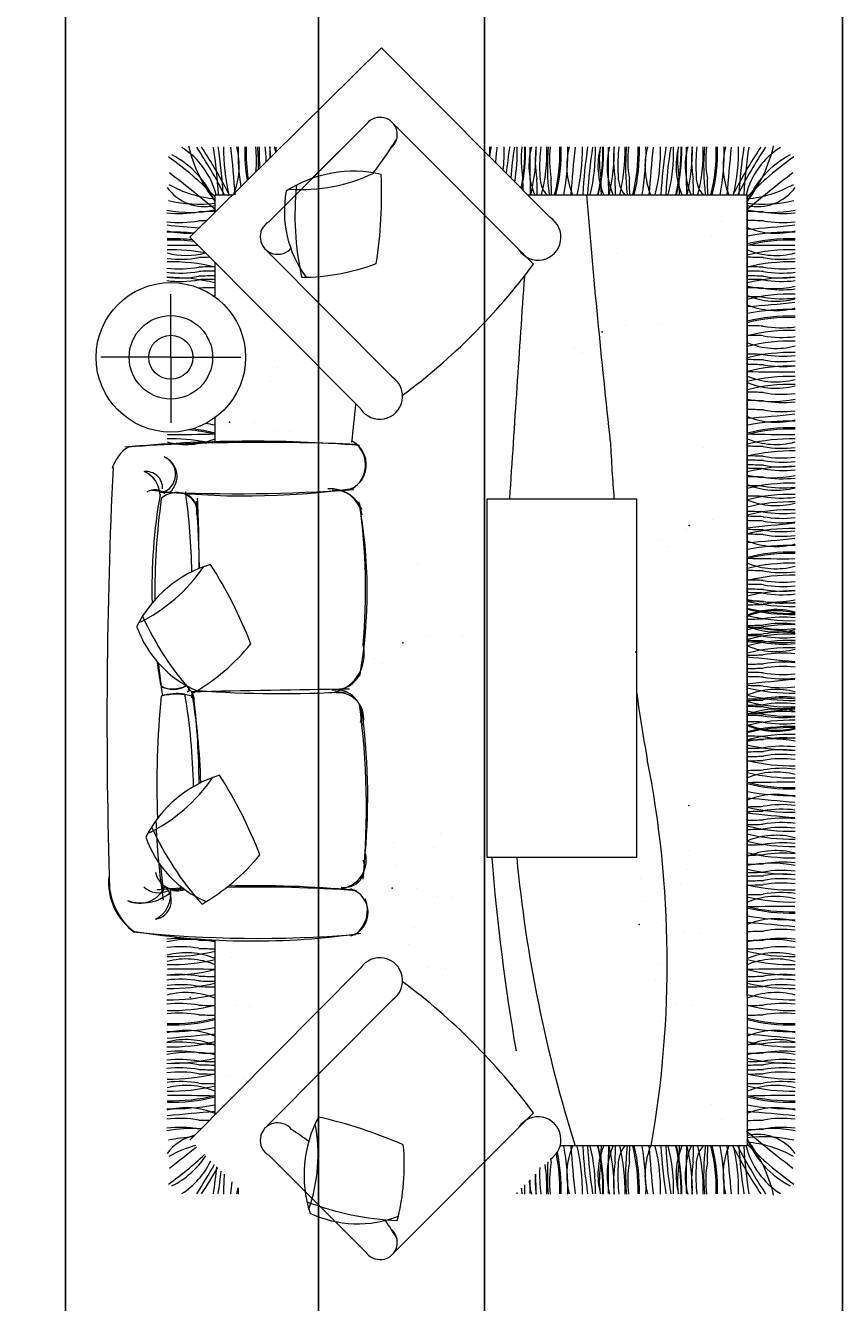
# Model space of a CAD drawing. Units: inches. Extents: x 338 to 1188, y -996 to 127.
# Tile 5 of 15: x 608 to 702, y -386 to -240. Entities that reach past the tile are written whole.
import ezdxf

# ---------------------------------------------------------------- set-up
doc = ezdxf.new("R2010")
doc.units = ezdxf.units.IN
doc.header["$MEASUREMENT"] = 0
doc.layers.add('A-ANNO-DIMS', color=5, linetype='Continuous', lineweight=18)
doc.layers.add('furniture', color=50, linetype='Continuous', lineweight=13, transparency=0.8)
doc.styles.get("Standard").update_dxf_attribs({"font": 'arial.ttf'})
doc.dimstyles.get("Standard").update_dxf_attribs({"dimtxt": 0.18, "dimasz": 0.18, "dimexe": 0.18, "dimexo": 0.0625, "dimgap": 0.09, "dimtad": 0, "dimtih": 1, "dimtoh": 1, "dimdec": 1, "dimzin": 0, "dimdsep": 46, "dimlunit": 4, "dimtxsty": 'Standard', "dimcen": 0.09, "dimadec": 0, "dimazin": 0, "dimtfac": 1, "dimtdec": 1, "dimtofl": 0, "dimtmove": 0, "dimatfit": 3, "dimfxl": 1, "dimtolj": 1, "dimtzin": 0, "dimarcsym": 0})

# ---------------------------------------------------------------- blocks, each defined once
blk = doc.blocks.new('*D31')
at = {"layer": 'A-ANNO-DIMS', "color": 0, "lineweight": -2, "transparency": 16777216}
for p, q in [((641.96, -149.3), (641.96, -968.86)), ((701.96, -149.3), (701.96, -968.86)), ((642.14, -968.68), (671.63, -968.68)), ((701.78, -968.68), (672.29, -968.68))]:
    blk.add_line(p, q, dxfattribs=at)
at = {"layer": 'A-ANNO-DIMS', "color": 0, "transparency": 16777216}
for points in [[(642.14, -968.65), (642.14, -968.71), (641.96, -968.68)], [(701.78, -968.65), (701.78, -968.71), (701.96, -968.68)]]:
    blk.add_solid(points, dxfattribs=at)
at = {"layer": 'Defpoints', "color": 0, "transparency": 16777216}
for p in [(641.96, -149.23), (701.96, -149.23), (701.96, -968.68)]:
    blk.add_point(p, dxfattribs=at)
at = {"layer": 'A-ANNO-DIMS', "color": 0, "transparency": 16777216, "insert": (671.96, -968.68), "char_height": 0.18, "attachment_point": 5}
blk.add_mtext('\\A1;5\'-0"', dxfattribs=at)
blk = doc.blocks.new('*D34')
at = {"layer": 'A-ANNO-DIMS', "color": 0, "lineweight": -2, "transparency": 16777216}
for p, q in [((612.96, -615.67), (612.96, 67.25)), ((613.14, 67.07), (636.63, 67.07)), ((660.78, 67.07), (637.3, 67.07)), ((660.96, -615.67), (660.96, 67.25))]:
    blk.add_line(p, q, dxfattribs=at)
at = {"layer": 'A-ANNO-DIMS', "color": 0, "transparency": 16777216}
for points in [[(613.14, 67.1), (613.14, 67.04), (612.96, 67.07)], [(660.78, 67.1), (660.78, 67.04), (660.96, 67.07)]]:
    blk.add_solid(points, dxfattribs=at)
at = {"layer": 'Defpoints', "color": 0, "transparency": 16777216}
for p in [(660.96, 67.07), (612.96, -615.73), (660.96, -615.73)]:
    blk.add_point(p, dxfattribs=at)
at = {"layer": 'A-ANNO-DIMS', "color": 0, "transparency": 16777216, "insert": (636.96, 67.07), "char_height": 0.18, "attachment_point": 5}
blk.add_mtext('\\A1;4\'-0"', dxfattribs=at)
blk = doc.blocks.new('*D48')
at = {"layer": 'A-ANNO-DIMS', "color": 0, "lineweight": -2, "transparency": 16777216}
for p, q in [((596.96, -615.67), (596.96, 67.25)), ((597.14, 67.07), (604.64, 67.07)), ((612.78, 67.07), (605.28, 67.07)), ((612.96, -615.67), (612.96, 67.25))]:
    blk.add_line(p, q, dxfattribs=at)
at = {"layer": 'A-ANNO-DIMS', "color": 0, "transparency": 16777216}
for points in [[(597.14, 67.1), (597.14, 67.04), (596.96, 67.07)], [(612.78, 67.1), (612.78, 67.04), (612.96, 67.07)]]:
    blk.add_solid(points, dxfattribs=at)
at = {"layer": 'Defpoints', "color": 0, "transparency": 16777216}
for p in [(612.96, 67.07), (596.96, -615.73), (612.96, -615.73)]:
    blk.add_point(p, dxfattribs=at)
at = {"layer": 'A-ANNO-DIMS', "color": 0, "transparency": 16777216, "insert": (604.96, 67.07), "char_height": 0.18, "attachment_point": 5}
blk.add_mtext('\\A1;1\'-4"', dxfattribs=at)

msp = doc.modelspace()

# ---------------------------------------------------------------- linework, layer by layer
at = {"layer": 'furniture'}
for p, q in [((627.21, -264.17), (649.14, -242.51)), ((649.14, -242.51), (668.47, -261.94)), ((636.25, -262.43), (647.5, -251.17)), ((641.22, -257.45), (647.5, -251.17)), ((666.56, -267.29), (650.39, -251.05)), ((664.92, -256.42), (664.92, -256.42)), ((664.96, -255.9), (664.96, -255.9)), ((673.87, -256.42), (673.87, -256.42)), ((673.91, -255.9), (673.91, -255.9)), ((682.82, -256.42), (682.82, -256.42)), ((682.86, -255.9), (682.86, -255.9)), ((630.09, -261.32), (630.09, -259.35)), ((630.09, -259.35), (632.09, -259.35)), ((665.89, -259.35), (691.05, -259.35)), ((691.05, -351.03), (691.05, -259.35)), ((691.05, -259.35), (691.05, -368.24)), ((628.37, -261.08), (628.37, -261.08)), ((628.37, -261.08), (628.37, -261.08)), ((628.37, -261.08), (628.37, -261.08)), ((636.25, -262.43), (638.05, -260.62)), ((692.76, -261.08), (692.76, -261.08)), ((692.76, -261.08), (692.76, -261.08)), ((692.76, -261.08), (692.76, -261.08)), ((628.7, -262.4), (628.7, -262.4)), ((628.7, -262.4), (628.7, -262.4)), ((628.7, -262.4), (628.7, -262.4)), ((688.07, -262.43), (688.07, -262.43)), ((692.44, -262.4), (692.44, -262.4)), ((692.44, -262.4), (692.44, -262.4)), ((692.44, -262.4), (692.44, -262.4)), ((627.21, -264.17), (646.78, -283.86)), ((686.91, -264.07), (686.91, -264.07)), ((635.85, -265.56), (650.41, -280.23)), ((676.07, -266.04), (676.07, -266.04)), ((630.09, -271.04), (630.09, -267.07)), ((625.03, -277.94), (625.03, -270.73)), ((677.16, -274.29), (677.16, -274.29)), ((681.22, -274.23), (681.22, -274.23)), ((674.17, -275.48), (674.17, -275.48)), ((671.23, -276.8), (671.23, -276.8)), ((671.23, -276.8), (671.23, -276.8)), ((672.13, -277.39), (672.13, -277.39)), ((672.13, -277.39), (672.13, -277.39)), ((625.03, -277.94), (617.01, -277.94)), ((625.03, -277.94), (633.05, -277.94)), ((625.03, -277.94), (625.03, -285.44)), ((637.29, -279.12), (637.29, -279.12)), ((636.5, -280.74), (636.5, -280.74)), ((630.09, -287.6), (630.09, -284.85)), ((631.37, -285.76), (631.37, -285.76)), ((634.56, -285.44), (634.56, -285.44)), ((636.93, -286.29), (636.93, -286.29)), ((638.59, -286.41), (638.59, -286.41)), ((686.04, -288.22), (686.04, -288.22)), ((661.25, -335.22), (661.25, -294.13)), ((661.25, -294.13), (678.37, -294.13)), ((678.37, -294.13), (678.37, -335.22)), ((687.13, -296.47), (687.13, -296.47)), ((691.19, -296.41), (691.19, -296.41)), ((684.14, -297.65), (684.14, -297.65)), ((681.2, -298.97), (681.2, -298.97)), ((681.2, -298.97), (681.2, -298.97)), ((682.09, -299.57), (682.09, -299.57)), ((682.09, -299.57), (682.09, -299.57)), ((653.25, -301.69), (653.25, -301.69)), ((692.76, -306.07), (692.76, -306.07)), ((692.76, -306.19), (692.76, -306.19)), ((654.33, -309.94), (654.33, -309.94)), ((658.39, -309.88), (658.39, -309.88)), ((692.76, -309.91), (692.76, -309.91)), ((651.35, -311.12), (651.35, -311.12)), ((648.41, -312.45), (648.41, -312.45)), ((648.41, -312.45), (648.41, -312.45)), ((649.3, -313.04), (649.3, -313.04)), ((649.3, -313.04), (649.3, -313.04)), ((692.76, -317.69), (692.76, -317.69)), ((692.76, -321.4), (692.76, -321.4)), ((692.76, -321.52), (692.76, -321.52)), ((655.93, -332.46), (655.93, -332.46)), ((650.58, -333.49), (650.58, -333.49)), ((655.15, -334.09), (655.15, -334.09)), ((684.27, -334.39), (684.27, -334.39)), ((650.8, -336.07), (650.8, -336.07)), ((678.37, -335.22), (661.25, -335.22)), ((678.87, -337.66), (678.87, -337.66)), ((684.23, -336.64), (684.23, -336.64)), ((650.01, -339.1), (650.01, -339.1)), ((653.21, -338.79), (653.21, -338.79)), ((683.44, -338.27), (683.44, -338.27)), ((655.58, -339.63), (655.58, -339.63)), ((657.23, -339.76), (657.23, -339.76)), ((679.09, -340.25), (679.09, -340.25)), ((652.89, -343.19), (652.89, -343.19)), ((678.31, -343.28), (678.31, -343.28)), ((681.5, -342.96), (681.5, -342.96)), ((630.09, -364.65), (630.09, -344.66)), ((632.79, -344.99), (632.79, -344.99)), ((683.87, -343.81), (683.87, -343.81)), ((685.53, -343.93), (685.53, -343.93)), ((627.43, -346.02), (627.43, -346.02)), ((652.21, -345.12), (652.21, -345.12)), ((627.21, -367.56), (646.78, -347.86)), ((632, -346.62), (632, -346.62)), ((654.54, -347.81), (654.54, -347.81)), ((656.47, -347.95), (656.47, -347.95)), ((681.18, -347.36), (681.18, -347.36)), ((627.65, -348.6), (627.65, -348.6)), ((680.5, -349.3), (680.5, -349.3)), ((652.67, -349.78), (652.67, -349.78)), ((652.67, -349.78), (652.67, -349.78)), ((626.86, -351.63), (626.86, -351.63)), ((630.06, -351.32), (630.06, -351.32)), ((632.43, -352.16), (632.43, -352.16)), ((634.09, -352.29), (634.09, -352.29)), ((635.85, -366.16), (650.41, -351.5)), ((682.83, -351.98), (682.83, -351.98)), ((684.76, -352.12), (684.76, -352.12)), ((680.97, -353.96), (680.97, -353.96)), ((680.97, -353.96), (680.97, -353.96)), ((629.74, -355.72), (629.74, -355.72)), ((629.06, -357.66), (629.06, -357.66)), ((631.39, -360.34), (631.39, -360.34)), ((633.32, -360.48), (633.32, -360.48)), ((629.53, -362.32), (629.53, -362.32)), ((629.53, -362.32), (629.53, -362.32)), ((686.91, -363.52), (686.91, -363.52)), ((628.7, -365.19), (628.7, -365.19)), ((628.7, -365.19), (628.7, -365.19)), ((628.7, -365.19), (628.7, -365.19)), ((666.56, -364.43), (650.39, -380.67)), ((688.07, -365.16), (688.07, -365.16)), ((692.44, -365.19), (692.44, -365.19)), ((692.44, -365.19), (692.44, -365.19)), ((692.44, -365.19), (692.44, -365.19)), ((628.37, -366.51), (628.37, -366.51)), ((628.37, -366.51), (628.37, -366.51)), ((628.37, -366.51), (628.37, -366.51)), ((692.76, -366.51), (692.76, -366.51)), ((692.76, -366.51), (692.76, -366.51)), ((692.76, -366.51), (692.76, -366.51)), ((691.05, -368.24), (669.63, -368.24)), ((636.25, -369.3), (647.5, -380.55)), ((636.25, -369.3), (640.41, -373.46)), ((673.87, -371.17), (673.87, -371.17)), ((682.82, -371.17), (682.82, -371.17)), ((673.91, -371.69), (673.91, -371.69)), ((682.86, -371.69), (682.86, -371.69)), ((643.84, -376.89), (647.5, -380.55))]:
    msp.add_line(p, q, dxfattribs=at)
for radius in [8.56, 4.78, 2.52]:
    msp.add_circle((625.03, -277.94), radius, dxfattribs=at)
for centre, radius, start, end in [((649, -252.44), 1.97, 310.1092, 139.8908), ((617.94, -233.04), 38.5, 321.8457, 328.9133), ((621.47, -261.52), 9.01, 13.9935, 57.7288), ((642.86, -250.08), 16.22, 192.9523, 218.0769), ((576.59, -287.48), 61.41, 27.2669, 33.1781), ((577.14, -287.47), 61.41, 27.2669, 33.1781), ((570.94, -262.81), 59.64, 3.3644, 8.6229), ((571.49, -262.8), 59.64, 3.3644, 8.6229), ((651.94, -254.34), 20.87, 178.6331, 193.8573), ((389.59, -278.5), 243.57, 4.5146, 5.8017), ((624.31, -256.05), 8.55, 337.3098, 14.8613), ((660.44, -254.32), 27.71, 179.0195, 188.4847), ((654.36, -254.35), 20.87, 178.6331, 189.2236), ((654.51, -254.35), 20.87, 178.6331, 188.8561), ((622.45, -255.33), 12.39, 353.6069, 6.8829), ((606.88, -256.06), 28.19, 359.2987, 4.5064), ((656, -254.35), 20.87, 178.6331, 185.2422), ((616.65, -256.01), 19.31, 1.4332, 6.4413), ((624.08, -255.33), 12.39, 1.3666, 6.8829), ((657.24, -254.34), 20.87, 178.6331, 182.1135), ((628.64, -256.03), 8.55, 10.6792, 14.8613), ((458.45, -255.12), 178.63, 0.2284, 0.3934), ((669.99, -256.05), 8.55, 165.1387, 172.5478), ((633.85, -254.32), 27.71, 358.619, 0.9805), ((904.7, -278.5), 243.57, 174.1983, 174.6171), ((642.35, -254.34), 20.87, 353.9229, 1.3669), ((722.8, -262.8), 59.64, 171.3771, 174.3194), ((723.35, -262.81), 59.64, 171.3771, 174.7986), ((643.84, -254.36), 20.87, 350.3159, 1.3669), ((644.71, -254.34), 20.87, 348.2362, 1.3669), ((677.55, -255.34), 12.39, 173.1171, 190.0651), ((644.78, -254.35), 20.87, 348.0993, 1.3669), ((674.6, -256.03), 8.55, 165.1387, 202.6902), ((844.78, -255.12), 178.63, 179.6066, 181.372), ((646, -254.34), 20.87, 346.1427, 1.3669), ((679.16, -255.33), 12.39, 173.1171, 190.0651), ((686.58, -256.01), 19.31, 173.5587, 182.5565), ((647.24, -254.35), 20.87, 346.1427, 1.3669), ((696.35, -256.06), 28.19, 175.4936, 186.6298), ((680.79, -255.33), 12.39, 173.1171, 190.0651), ((648.73, -254.35), 20.87, 346.1427, 1.3669), ((648.88, -254.35), 20.87, 346.1427, 1.3669), ((642.8, -254.32), 27.71, 349.5961, 0.9805), ((678.93, -256.05), 8.55, 165.1387, 202.6902), ((913.65, -278.5), 243.57, 174.1983, 175.4854), ((651.3, -254.34), 20.87, 346.1427, 1.3669), ((731.74, -262.8), 59.64, 171.3771, 176.6356), ((732.3, -262.81), 59.64, 171.3771, 176.6356), ((652.8, -254.36), 20.87, 346.1427, 1.3669), ((653.66, -254.34), 20.87, 346.1427, 1.3669), ((682.5, -256.05), 8.55, 165.1387, 202.6902), ((653.73, -254.35), 20.87, 346.1427, 1.3669), ((686.5, -255.34), 12.39, 173.1171, 190.0651), ((683.55, -256.03), 8.55, 165.1387, 202.6902), ((853.74, -255.12), 178.63, 179.6066, 181.372), ((654.96, -254.34), 20.87, 346.1427, 1.3669), ((688.12, -255.33), 12.39, 173.1171, 190.0651), ((695.54, -256.01), 19.31, 173.5587, 182.5565), ((656.19, -254.35), 20.87, 346.1427, 1.3669), ((705.31, -256.06), 28.19, 175.4936, 186.6298), ((689.75, -255.33), 12.39, 173.1171, 190.0651), ((657.68, -254.35), 20.87, 346.1427, 1.3669), ((657.84, -254.35), 20.87, 346.1427, 1.3669), ((651.75, -254.32), 27.71, 349.5961, 0.9805), ((687.89, -256.05), 8.55, 165.1387, 202.6902), ((922.6, -278.5), 243.57, 174.1983, 175.4854), ((660.25, -254.34), 20.87, 346.1427, 1.3669), ((740.7, -262.8), 59.64, 171.3771, 176.6356), ((741.25, -262.81), 59.64, 171.3771, 176.6356), ((661.74, -254.36), 20.87, 346.1427, 1.3669), ((662.61, -254.34), 20.87, 346.1427, 1.3669), ((691.45, -256.05), 8.55, 165.1387, 202.6902), ((662.68, -254.35), 20.87, 346.1427, 1.3669), ((695.45, -255.34), 12.39, 173.1171, 190.0651), ((692.5, -256.03), 8.55, 165.1387, 202.6902), ((862.68, -255.12), 178.63, 179.6066, 181.372), ((663.9, -254.34), 20.87, 346.1427, 1.3669), ((697.06, -255.33), 12.39, 173.1171, 190.0651), ((704.48, -256.01), 19.31, 173.5587, 182.5565), ((665.14, -254.35), 20.87, 346.1427, 1.3669), ((714.25, -256.06), 28.19, 175.4936, 186.6298), ((698.69, -255.33), 12.39, 173.1171, 190.0651), ((666.63, -254.35), 20.87, 346.1427, 1.3669), ((666.78, -254.35), 20.87, 346.1427, 1.3669), ((660.7, -254.32), 27.71, 349.5961, 0.9805), ((696.83, -256.05), 8.55, 165.1387, 202.6902), ((931.54, -278.5), 243.57, 174.1983, 175.4854), ((744, -287.47), 61.41, 146.8219, 152.7331), ((669.2, -254.34), 20.87, 346.1427, 1.3669), ((744.55, -287.48), 61.41, 146.8219, 152.7331), ((749.64, -262.8), 59.64, 171.3771, 176.6356), ((750.2, -262.81), 59.64, 171.3771, 176.6356), ((699.67, -261.52), 9.01, 122.2712, 166.0065), ((678.27, -250.08), 16.22, 321.9231, 347.0477), ((603.49, -285.02), 36.8, 43.716, 54.6847), ((620.32, -264.15), 10.55, 22.1181, 62.6967), ((700.82, -264.15), 10.55, 117.3033, 157.8819), ((717.65, -285.02), 36.8, 125.3153, 136.284), ((521.87, -390.83), 169.01, 50.1568, 52.4559), ((645.94, -270.78), 14.14, 77.0126, 122.9429), ((640, -239.59), 19.14, 265.9005, 295.6513), ((596.23, -259.24), 52.94, 351.3371, 2.4176), ((671.02, -257.08), 3.73, 176.8256, 218.3436), ((679.98, -257.08), 3.73, 176.8256, 218.3436), ((688.92, -257.08), 3.73, 176.8256, 218.3436), ((799.27, -390.83), 169.01, 127.5441, 129.8432), ((628.91, -255.36), 5.33, 215.9057, 282.8054), ((631.03, -247.3), 12.51, 240.135, 265.7243), ((672.65, -261.68), 33.41, 174.0815, 192.2768), ((527.26, -261.87), 138.16, 1.2535, 1.8109), ((528.87, -261.86), 138.16, 1.0225, 1.8109), ((530.5, -261.86), 138.16, 1.0225, 1.8109), ((536.21, -261.87), 138.16, 1.0225, 1.8109), ((537.83, -261.86), 138.16, 1.0225, 1.8109), ((539.46, -261.86), 138.16, 1.0225, 1.8109), ((545.16, -261.87), 138.16, 1.0225, 1.8109), ((546.77, -261.86), 138.16, 1.0225, 1.8109), ((548.4, -261.86), 138.16, 1.0225, 1.8109), ((690.11, -247.3), 12.51, 274.2757, 299.865), ((692.23, -255.36), 5.33, 257.1946, 324.0943), ((628.22, -245.35), 15.05, 256.7215, 277.1491), ((650.65, -261.22), 12.62, 169.4501, 216.7699), ((1680.39, -176.52), 1011.15, 184.69873, 186.31076), ((692.92, -245.35), 15.05, 262.8509, 283.2785), ((626.07, -249.09), 12.39, 263.1171, 280.0651), ((627.29, -247.47), 13.88, 258.7545, 281.5888), ((632.6, -399.38), 138.16, 91.0225, 91.8109), ((688.54, -399.38), 138.16, 88.1891, 88.9775), ((693.84, -247.47), 13.88, 258.4112, 281.2455), ((695.07, -249.09), 12.39, 259.9349, 276.8829), ((626.06, -250.12), 12.39, 263.1171, 280.0651), ((649.24, -20.47), 243.57, 264.1983, 265.0575), ((632.6, -400.41), 138.16, 91.4616, 91.8109), ((637.26, -264.15), 2, 120.4819, 322.3252), ((667.09, -264.19), 2.63, 213.0924, 58.5307), ((688.54, -400.41), 138.16, 88.1891, 88.9775), ((694.34, -255.18), 8.55, 247.3098, 284.8613), ((671.9, -20.47), 243.57, 274.5146, 275.8017), ((695.07, -250.12), 12.39, 259.9349, 276.8829), ((625.06, -291.32), 27.71, 84.6488, 90.9805), ((626.8, -255.18), 8.55, 255.1387, 276.0041), ((625.1, -285.23), 20.87, 83.2584, 91.3669), ((625.09, -285.39), 20.87, 82.7707, 91.3669), ((696.04, -285.23), 20.87, 88.6331, 103.8573), ((696.04, -285.39), 20.87, 88.6331, 103.8573), ((696.07, -291.32), 27.71, 89.0195, 100.4039), ((625.09, -286.5), 20.87, 79.2534, 91.3669), ((626.79, -257.73), 8.55, 255.1387, 284.8341), ((625.87, -86.49), 178.63, 269.6066, 270.7304), ((695.27, -86.49), 178.63, 268.628, 270.3934), ((694.35, -257.73), 8.55, 247.3098, 284.8613), ((696.05, -286.5), 20.87, 88.6331, 103.8573), ((626.08, -254.33), 12.39, 263.1171, 280.0651), ((625.09, -287.88), 20.87, 76.1427, 91.3669), ((632.61, -404.62), 138.16, 91.2964, 91.8109), ((639.87, -244.04), 24.74, 270.3068, 290.5663), ((608.1, -223.87), 72.82, 306.6613, 323.3951), ((688.53, -404.62), 138.16, 88.1891, 88.9775), ((696.05, -287.88), 20.87, 88.6331, 103.8573), ((695.06, -254.33), 12.39, 259.9349, 276.8829), ((626.07, -255.42), 12.39, 263.1171, 280.0651), ((626.07, -255.91), 12.39, 263.1171, 280.0651), ((626.07, -256.46), 12.39, 263.1171, 280.0651), ((625.08, -289.68), 20.87, 76.1427, 91.3669), ((632.6, -405.71), 138.16, 91.0225, 91.8109), ((632.6, -406.2), 138.16, 91.0225, 91.8109), ((632.6, -406.75), 138.16, 91.0225, 91.8109), ((5549.12, -607.42), 4895.33, 176.03178, 176.33069), ((688.53, -405.71), 138.16, 88.1891, 88.9775), ((688.54, -406.2), 138.16, 88.1891, 88.9775), ((688.54, -406.75), 138.16, 88.1891, 88.9775), ((696.05, -289.68), 20.87, 88.6331, 103.8573), ((695.06, -255.42), 12.39, 259.9349, 276.8829), ((695.07, -255.91), 12.39, 259.9349, 276.8829), ((695.07, -256.46), 12.39, 259.9349, 276.8829), ((626.07, -256.86), 12.39, 263.1171, 280.0651), ((632.6, -407.15), 138.16, 91.0225, 91.8109), ((632.6, -408.11), 138.16, 91.0225, 91.8109), ((688.54, -407.15), 138.16, 88.1891, 88.9775), ((688.54, -408.11), 138.16, 88.1891, 88.9775), ((693.84, -256.2), 13.88, 258.4112, 281.2455), ((695.07, -256.86), 12.39, 259.9349, 276.8829), ((695.07, -257.82), 12.39, 259.9349, 276.8829), ((626.78, -262.98), 8.55, 291.652, 292.6902), ((632.6, -409.14), 138.16, 91.0225, 91.0606), ((688.54, -409.14), 138.16, 88.1891, 88.9775), ((694.34, -264.03), 8.55, 247.3098, 284.8613), ((696.06, -291.57), 20.87, 88.6331, 103.8573), ((694.36, -262.98), 8.55, 247.3098, 284.8613), ((671.9, -29.32), 243.57, 274.5146, 275.8017), ((695.07, -258.85), 12.39, 259.9349, 276.8829), ((696.04, -294.08), 20.87, 88.6331, 103.8573), ((696.04, -294.24), 20.87, 88.6331, 103.8573), ((696.07, -300.17), 27.71, 89.0195, 100.4039), ((688.53, -412.46), 138.16, 88.1891, 88.9775), ((695.06, -262.17), 12.39, 259.9349, 276.8829), ((688.53, -413.56), 138.16, 88.1891, 88.9775), ((696.05, -295.73), 20.87, 88.6331, 103.8573), ((696.06, -296.96), 20.87, 88.6331, 103.8573), ((694.36, -268.37), 8.55, 247.3098, 284.8613), ((695.06, -263.27), 12.39, 259.9349, 276.8829), ((688.52, -415.71), 138.16, 88.1891, 88.9775), ((696.06, -298.26), 20.87, 88.6331, 103.8573), ((695.06, -265.42), 12.39, 259.9349, 276.8829), ((688.54, -416.34), 138.16, 88.1891, 88.9775), ((688.54, -416.89), 138.16, 88.1891, 88.9775), ((696.05, -299.82), 20.87, 88.6331, 103.8573), ((695.07, -266.05), 12.39, 259.9349, 276.8829), ((695.07, -266.6), 12.39, 259.9349, 276.8829), ((648.96, -282.41), 2.62, 213.6335, 56.3665), ((695.27, -100.98), 178.63, 268.628, 270.3934), ((694.35, -272.21), 8.55, 247.3098, 284.8613), ((696.05, -300.99), 20.87, 88.6331, 103.8573), ((688.54, -420.06), 138.16, 88.1891, 88.9775), ((694.34, -272.93), 8.55, 247.3098, 284.8613), ((696.04, -301.92), 20.87, 88.6331, 103.8573), ((695.07, -269.78), 12.39, 259.9349, 276.8829), ((-359.26, -176.52), 1011.15, 353.68924, 353.93736), ((688.54, -421.02), 138.16, 88.1891, 88.9775), ((693.84, -269.12), 13.88, 258.4112, 281.2455), ((695.07, -270.73), 12.39, 259.9349, 276.8829), ((688.54, -422.05), 138.16, 88.1891, 88.9775), ((694.34, -276.83), 8.55, 247.3098, 284.8613), ((671.9, -42.11), 243.57, 274.5146, 275.8017), ((695.07, -271.77), 12.39, 259.9349, 276.8829), ((625.09, -307.03), 20.87, 76.1427, 84.5854), ((625.1, -306.88), 20.87, 76.1427, 83.4467), ((625.06, -312.96), 27.71, 79.5961, 81.862), ((696.04, -306.88), 20.87, 88.6331, 103.8573), ((696.04, -307.03), 20.87, 88.6331, 103.8573), ((696.07, -312.96), 27.71, 89.0195, 100.4039), ((634.36, -441.94), 154.39, 85.4325, 95.431), ((635.72, -514.28), 226.6, 87.3143, 93.933), ((626.79, -279.37), 8.55, 255.1387, 292.6902), ((625.09, -308.15), 20.87, 79.3731, 91.3669), ((625.87, -108.14), 178.63, 269.6066, 271.372), ((644.39, -290.24), 3.03, 284.6379, 64.3095), ((644.1, -290.25), 3.23, 303.041, 46.0653), ((894.28, -277.01), 219.16, 182.7877, 184.4807), ((695.27, -108.14), 178.63, 268.628, 270.3934), ((694.35, -279.37), 8.55, 247.3098, 284.8613), ((696.05, -308.15), 20.87, 88.6331, 103.8573), ((622.46, -291.88), 4.32, 121.8817, 163.9672), ((623.43, -291.34), 2.15, 284.7814, 67.5922), ((623.33, -291.58), 2.41, 312.3134, 67.6102), ((688.53, -426.26), 138.16, 88.1891, 88.9775), ((688.53, -427.36), 138.16, 88.1891, 88.9775), ((696.05, -309.53), 20.87, 88.6331, 103.8573), ((695.06, -275.97), 12.39, 259.9349, 276.8829), ((695.06, -277.07), 12.39, 259.9349, 276.8829), ((1229.86, -319.71), 612.15, 177.2697, 181.7875), ((688.54, -427.85), 138.16, 88.1891, 88.9775), ((688.54, -428.39), 138.16, 88.1891, 88.9775), ((688.54, -428.79), 138.16, 88.1891, 88.9775), ((696.05, -311.32), 20.87, 88.6331, 103.8573), ((695.07, -277.56), 12.39, 259.9349, 276.8829), ((695.07, -278.1), 12.39, 259.9349, 276.8829), ((695.07, -278.51), 12.39, 259.9349, 276.8829), ((622.19, -292.92), 1.9, 358.0108, 96.5585), ((620.89, -293.69), 2.87, 1.184, 67.8216), ((688.54, -429.75), 138.16, 88.1891, 88.9775), ((693.84, -277.85), 13.88, 258.4112, 281.2455), ((696.06, -313.22), 20.87, 88.6331, 103.8573), ((695.07, -279.46), 12.39, 259.9349, 276.8829), ((623.19, -294.72), 1.62, 44.3938, 123.5856), ((633.58, -205.5), 88.31, 262.9836, 277.989), ((684.53, -304.37), 61.67, 169.9466, 181.5903), ((632.28, -95.63), 197.93, 267.5073, 273.9592), ((625.66, -295.95), 2.52, 6.1174, 133.1189), ((626, -295.47), 2, 347.6226, 80.3094), ((540.68, -304.58), 86.78, 1.3731, 7.4472), ((643.33, -296.69), 3.7, 10.9756, 94.9747), ((643.67, -296.58), 3.43, 19.8228, 92.4985), ((688.52, -431.96), 138.16, 88.1891, 88.9775), ((688.54, -430.78), 138.16, 88.1891, 88.9775), ((694.36, -284.62), 8.55, 247.3098, 284.8613), ((696.06, -314.51), 20.87, 88.6331, 103.8573), ((695.07, -280.5), 12.39, 259.9349, 276.8829), ((702.53, -304.94), 79.34, 172.1551, 180.5585), ((509.53, -303.66), 118.78, 0.7456, 4.456), ((480.55, -301.19), 147.71, 359.6386, 2.7653), ((591.12, -304.69), 56.4, 350.0543, 10.4167), ((572.03, -304.61), 75.3, 355.2072, 7.551), ((694.34, -286.37), 8.55, 247.3098, 284.8613), ((696.04, -315.36), 20.87, 88.6331, 103.8573), ((695.06, -281.67), 12.39, 259.9349, 276.8829), ((688.52, -433.73), 138.16, 88.1891, 88.9775), ((688.53, -434.28), 138.16, 88.1891, 88.9775), ((688.54, -434.78), 138.16, 88.1891, 88.9775), ((696.04, -316.27), 20.87, 88.6331, 103.8573), ((695.05, -283.44), 12.39, 259.9349, 276.8829), ((695.06, -283.99), 12.39, 259.9349, 276.8829), ((695.07, -284.49), 12.39, 259.9349, 276.8829), ((688.51, -435.8), 138.16, 88.1891, 88.9775), ((688.52, -436.33), 138.16, 88.1891, 88.9775), ((739.31, -758.16), 463.19, 95.3008, 95.9835), ((696.03, -318.42), 20.87, 88.6331, 103.8573), ((695.04, -285.51), 12.39, 259.9349, 276.8829), ((695.05, -286.04), 12.39, 259.9349, 276.8829), ((694.34, -291.05), 8.55, 247.3098, 284.8613), ((671.9, -56.34), 243.57, 274.5146, 275.8017), ((696.07, -327.19), 27.71, 89.0195, 100.4039), ((695.27, -122.37), 178.63, 268.628, 270.3934), ((696.04, -321.11), 20.87, 88.6331, 103.8573), ((696.04, -321.26), 20.87, 88.6331, 103.8573), ((633.71, -315.17), 14.14, 107.0126, 152.9429), ((612.97, -291.13), 19.14, 295.9005, 325.6513), ((584.89, -330.03), 52.94, 21.3371, 32.4176), ((688.53, -440.49), 138.16, 88.1891, 88.9775), ((694.35, -293.6), 8.55, 247.3098, 284.8613), ((696.05, -322.38), 20.87, 88.6331, 103.8573), ((695.06, -290.2), 12.39, 259.9349, 276.8829), ((688.53, -441.58), 138.16, 88.1891, 88.9775), ((688.54, -442.07), 138.16, 88.1891, 88.9775), ((696.05, -323.76), 20.87, 88.6331, 103.8573), ((695.06, -291.3), 12.39, 259.9349, 276.8829), ((695.07, -291.79), 12.39, 259.9349, 276.8829), ((688.54, -442.62), 138.16, 88.1891, 88.9775), ((688.54, -443.02), 138.16, 88.1891, 88.9775), ((696.05, -325.55), 20.87, 88.6331, 103.8573), ((695.07, -292.33), 12.39, 259.9349, 276.8829), ((695.07, -292.74), 12.39, 259.9349, 276.8829), ((688.52, -168.14), 138.16, 271.0225, 271.8109), ((688.54, -443.98), 138.16, 88.1891, 88.9775), ((696.04, -285.6), 20.87, 256.1427, 271.3669), ((696.04, -286.39), 20.87, 256.1427, 271.3669), ((696.04, -286.51), 20.87, 256.1427, 271.3669), ((694.34, -315.38), 8.55, 75.1387, 112.6902), ((694.34, -315.5), 8.55, 75.1387, 112.6902), ((693.84, -292.08), 13.88, 258.4112, 281.2455), ((695.05, -318.42), 12.39, 83.1171, 100.0651), ((695.07, -293.69), 12.39, 259.9349, 276.8829), ((652.29, -293.94), 33.41, 204.0815, 222.2768), ((688.52, -169.79), 138.16, 271.0225, 271.8109), ((696.06, -287.23), 20.87, 256.1427, 271.3669), ((695.04, -320.8), 12.39, 83.1171, 100.0651), ((695.06, -320.08), 12.39, 83.1171, 100.0651), ((633.01, -304.54), 12.62, 199.4501, 246.7699), ((688.51, -170.51), 138.16, 271.0225, 271.8109), ((688.52, -447.96), 138.16, 88.1891, 88.9775), ((688.54, -446.99), 138.16, 88.1891, 88.9775), ((688.54, -171.53), 138.16, 271.0225, 271.8109), ((739.31, 151.84), 463.19, 264.0165, 264.6992), ((696.04, -330.5), 20.87, 88.6331, 103.8573), ((696.06, -329.42), 20.87, 88.6331, 103.8573), ((694.36, -300.83), 8.55, 247.3098, 284.8613), ((695.05, -297.67), 12.39, 259.9349, 276.8829), ((695.07, -296.7), 12.39, 259.9349, 276.8829), ((695.07, -321.82), 12.39, 83.1171, 100.0651), ((615.08, -295.05), 24.74, 300.3068, 320.5663), ((642.73, -311.94), 4.46, 276.5867, 13.4511), ((688.53, -448.51), 138.16, 88.1891, 88.9775), ((688.52, -448.67), 138.16, 88.1891, 88.9775), ((694.34, -303.09), 8.55, 247.3098, 284.8613), ((696.04, -332.07), 20.87, 88.6331, 103.8573), ((696.06, -331.23), 20.87, 88.6331, 103.8573), ((695.06, -298.22), 12.39, 259.9349, 276.8829), ((695.06, -298.39), 12.39, 259.9349, 276.8829), ((684.53, -304.37), 61.67, 187.803, 190.4557), ((688.51, -173.92), 138.16, 271.0225, 271.8109), ((739.31, 148.44), 463.19, 264.0165, 264.6992), ((695.04, -324.21), 12.39, 83.1171, 100.0651), ((695.07, -325.23), 12.39, 83.1171, 100.0651), ((702.53, -304.94), 79.34, 185.7795, 188.522), ((643.77, -312.77), 3.26, 264.9234, 335.6374), ((688.53, -175.44), 138.16, 271.0225, 271.8109), ((688.53, -452.15), 138.16, 88.1891, 88.9775), ((688.54, -174.94), 138.16, 271.0225, 271.8109), ((695.06, -325.73), 12.39, 83.1171, 100.0651), ((695.06, -301.87), 12.39, 259.9349, 276.8829), ((625.35, -313.1), 2.86, 239.8319, 299.468), ((625.14, -311.68), 4.21, 253.3108, 292.6164), ((540.68, -304.58), 86.78, 352.7245, 352.7726), ((688.51, -453.67), 138.16, 88.1891, 88.9775), ((688.54, -452.65), 138.16, 88.1891, 88.9775), ((739.31, -776.03), 463.19, 95.3008, 95.9835), ((696.04, -295.52), 20.87, 256.1427, 271.3669), ((695.04, -303.38), 12.39, 259.9349, 276.8829), ((695.07, -302.37), 12.39, 259.9349, 276.8829), ((726.88, -326.9), 103.45, 174.3639, 182.1219), ((625.66, -323.59), 7.07, 74.0479, 104.2061), ((625.78, -322.25), 5.81, 81.5362, 108.3493), ((556.66, -328.34), 70.97, 1.0061, 9.6001), ((626.03, -314.7), 1.79, 299.1313, 312.0141), ((637.67, -184.19), 132.26, 265.3655, 265.4784), ((27526.63, -1508420.89), 1508344.52, 91.02115817, 91.0218453), ((480.55, -301.19), 147.71, 353.8872, 354.1215), ((552.71, -328.82), 75.78, 1.6458, 9.5268), ((656.61, -307.96), 30.31, 195.9625, 197.4638), ((532.99, -327.56), 95.28, 0.4949, 6.3291), ((637.67, -184.19), 132.26, 265.8425, 273.2873), ((644.03, -318.89), 2.86, 343.4437, 91.8228), ((644.24, -319.24), 2.88, 342.9316, 95.1092), ((908.76, -283.39), 232.73, 188.119, 190.0442), ((688.52, -178.92), 138.16, 271.0225, 271.8109), ((688.53, -179.09), 138.16, 271.0225, 271.8109), ((694.34, -324.51), 8.55, 75.1387, 112.6902), ((696.06, -296.36), 20.87, 256.1427, 271.3669), ((695.06, -329.2), 12.39, 83.1171, 100.0651), ((695.06, -329.37), 12.39, 83.1171, 100.0651), ((558.01, -329.61), 89.42, 354.8245, 7.7148), ((571.86, -328.22), 75.72, 355.0781, 7.695), ((688.52, -179.63), 138.16, 271.0225, 271.8109), ((688.54, -456.06), 138.16, 88.1891, 88.9775), ((688.54, -180.6), 138.16, 271.0225, 271.8109), ((739.31, -779.44), 463.19, 95.3008, 95.9835), ((696.04, -297.1), 20.87, 256.1427, 271.3669), ((694.36, -326.76), 8.55, 75.1387, 112.6902), ((696.06, -298.17), 20.87, 256.1427, 271.3669), ((695.05, -329.92), 12.39, 83.1171, 100.0651), ((695.07, -305.77), 12.39, 259.9349, 276.8829), ((695.07, -330.89), 12.39, 83.1171, 100.0651), ((688.51, -457.08), 138.16, 88.1891, 88.9775), ((688.52, -457.8), 138.16, 88.1891, 88.9775), ((694.34, -312.09), 8.55, 247.3098, 284.8613), ((694.34, -312.21), 8.55, 247.3098, 284.8613), ((696.06, -340.36), 20.87, 88.6331, 103.8573), ((695.04, -306.79), 12.39, 259.9349, 276.8829), ((695.06, -307.52), 12.39, 259.9349, 276.8829), ((688.52, -459.45), 138.16, 88.1891, 88.9775), ((696.04, -341.08), 20.87, 88.6331, 103.8573), ((696.04, -341.2), 20.87, 88.6331, 103.8573), ((696.04, -341.99), 20.87, 88.6331, 103.8573), ((695.05, -309.17), 12.39, 259.9349, 276.8829), ((695.07, -333.9), 12.39, 83.1171, 100.0651), ((688.54, -184.57), 138.16, 271.0225, 271.8109), ((688.54, -184.97), 138.16, 271.0225, 271.8109), ((688.54, -183.61), 138.16, 271.0225, 271.8109), ((693.84, -335.52), 13.88, 78.7545, 101.5888), ((696.05, -302.04), 20.87, 256.1427, 271.3669), ((695.07, -334.86), 12.39, 83.1171, 100.0651), ((695.07, -335.26), 12.39, 83.1171, 100.0651), ((562.11, -347.29), 119.78, 349.9275, 11.2246), ((688.54, -185.52), 138.16, 271.0225, 271.8109), ((688.53, -186.01), 138.16, 271.0225, 271.8109), ((696.05, -303.84), 20.87, 256.1427, 271.3669), ((695.07, -335.8), 12.39, 83.1171, 100.0651), ((695.06, -336.29), 12.39, 83.1171, 100.0651), ((634.75, -339.3), 14.14, 107.0126, 152.9429), ((585.92, -354.16), 52.94, 21.3371, 32.4176), ((688.53, -187.1), 138.16, 271.0225, 271.8109), ((694.35, -333.99), 8.55, 75.1387, 112.6902), ((696.05, -305.22), 20.87, 256.1427, 271.3669), ((695.06, -337.39), 12.39, 83.1171, 100.0651), ((614.01, -315.26), 19.14, 295.9005, 325.6513), ((695.27, -505.23), 178.63, 89.6066, 91.372), ((696.04, -306.33), 20.87, 256.1427, 271.3669), ((696.04, -306.49), 20.87, 256.1427, 271.3669), ((694.34, -336.54), 8.55, 75.1387, 112.6902), ((696.07, -300.4), 27.71, 259.5961, 270.9805), ((671.9, -571.25), 243.57, 84.1983, 85.4854), ((688.51, -191.8), 138.16, 271.0225, 271.8109), ((688.52, -191.26), 138.16, 271.0225, 271.8109), ((739.31, 130.56), 463.19, 264.0165, 264.6992), ((696.03, -309.17), 20.87, 256.1427, 271.3669), ((695.04, -342.08), 12.39, 83.1171, 100.0651), ((695.05, -341.55), 12.39, 83.1171, 100.0651), ((653.33, -318.07), 33.41, 204.0815, 222.2768), ((709.07, -327.69), 85.83, 182.2017, 188.3067), ((688.53, -193.31), 138.16, 271.0225, 271.8109), ((688.54, -192.81), 138.16, 271.0225, 271.8109), ((696.04, -311.33), 20.87, 256.1427, 271.3669), ((695.06, -343.6), 12.39, 83.1171, 100.0651), ((695.05, -344.15), 12.39, 83.1171, 100.0651), ((695.07, -343.1), 12.39, 83.1171, 100.0651), ((634.05, -328.67), 12.62, 199.4501, 246.7699), ((688.52, -193.86), 138.16, 271.0225, 271.8109), ((696.04, -312.24), 20.87, 256.1427, 271.3669), ((694.34, -341.22), 8.55, 75.1387, 112.6902), ((644.12, -335.51), 3.29, 267.6579, 14.0974), ((688.52, -195.63), 138.16, 271.0225, 271.8109), ((696.06, -313.08), 20.87, 256.1427, 271.3669), ((694.36, -342.97), 8.55, 75.1387, 112.6902), ((696.06, -314.38), 20.87, 256.1427, 271.3669), ((695.06, -345.92), 12.39, 83.1171, 100.0651), ((695.07, -347.1), 12.39, 83.1171, 100.0651), ((726.88, -326.9), 103.45, 185.0871, 186.7491), ((616.12, -319.19), 24.74, 300.3068, 320.5663), ((644.94, -336.35), 2.28, 260.2617, 21.0115), ((909.91, -315.17), 248.94, 184.6196, 189.7513), ((824.58, -319.98), 160.66, 185.4421, 197.4799), ((688.54, -196.81), 138.16, 271.0225, 271.8109), ((688.54, -197.84), 138.16, 271.0225, 271.8109), ((693.84, -349.74), 13.88, 78.7545, 101.5888), ((695.07, -348.13), 12.39, 83.1171, 100.0651), ((624.59, -338.13), 6.69, 173.8792, 237.1093), ((625.66, -336.46), 2.42, 190.6216, 289.193), ((688.54, -198.8), 138.16, 271.0225, 271.8109), ((688.54, -199.2), 138.16, 271.0225, 271.8109), ((696.05, -316.27), 20.87, 256.1427, 271.3669), ((695.07, -349.08), 12.39, 83.1171, 100.0651), ((695.07, -349.49), 12.39, 83.1171, 100.0651), ((695.07, -350.03), 12.39, 83.1171, 100.0651), ((626.1, -337.57), 8.18, 188.6549, 228.7104), ((621.43, -337.27), 3.18, 244.8715, 336.7247), ((621.69, -335.39), 5.03, 251.2473, 311.1348), ((623.63, -336.7), 2.54, 227.7203, 294.4461), ((622.93, -340.16), 2.15, 279.2916, 47.6289), ((621.75, -339.39), 3.28, 297.8433, 9.8684), ((634.54, -464.2), 125.76, 93.7101, 95.0653), ((625.79, -336.85), 2.17, 237.7366, 292.2387), ((635.09, -491.45), 152.85, 93.1908, 93.7892), ((635.09, -491.45), 152.85, 85.8027, 91.3803), ((634.54, -464.2), 125.76, 84.7422, 91.3335), ((644.8, -341.5), 2.82, 287.7157, 72.8428), ((688.54, -199.75), 138.16, 271.0225, 271.8109), ((688.53, -200.24), 138.16, 271.0225, 271.8109), ((696.05, -318.06), 20.87, 256.1427, 271.3669), ((695.06, -350.52), 12.39, 83.1171, 100.0651), ((644.14, -341.26), 3.41, 306.0678, 22.6723), ((688.53, -201.33), 138.16, 271.0225, 271.8109), ((694.35, -348.22), 8.55, 75.1387, 112.6902), ((696.05, -319.44), 20.87, 256.1427, 271.3669), ((695.06, -351.62), 12.39, 83.1171, 100.0651), ((695.27, -519.45), 178.63, 89.6066, 91.372), ((696.04, -320.56), 20.87, 256.1427, 271.3669), ((696.04, -320.71), 20.87, 256.1427, 271.3669), ((696.07, -314.63), 27.71, 259.5961, 270.9805), ((694.34, -350.77), 8.55, 75.1387, 112.6902), ((671.9, -585.48), 243.57, 84.1983, 85.4854), ((695.07, -355.83), 12.39, 83.1171, 100.0651), ((635, -206.2), 138.27, 264.0627, 274.6253), ((634.44, -259.7), 85.07, 260.8079, 278.3514), ((626.07, -356.86), 12.39, 79.9349, 96.8829), ((627.29, -358.47), 13.88, 78.4112, 101.2455), ((632.6, -206.57), 138.16, 268.1891, 268.9775), ((688.54, -205.54), 138.16, 271.0225, 271.8109), ((688.54, -206.57), 138.16, 271.0225, 271.8109), ((693.84, -358.47), 13.88, 78.7545, 101.5888), ((695.07, -356.86), 12.39, 83.1171, 100.0651), ((626.07, -357.81), 12.39, 79.9349, 96.8829), ((625.1, -325.67), 20.87, 268.6331, 283.8573), ((626.8, -354.66), 8.55, 67.3098, 104.8613), ((632.6, -207.53), 138.16, 268.1891, 268.9775), ((688.54, -207.53), 138.16, 271.0225, 271.8109), ((696.04, -325.67), 20.87, 256.1427, 271.3669), ((694.34, -354.66), 8.55, 75.1387, 112.6902), ((695.07, -357.81), 12.39, 83.1171, 100.0651), ((626.79, -355.38), 8.55, 67.3098, 104.8613), ((625.09, -326.61), 20.87, 268.6331, 283.8573), ((648.96, -349.31), 2.62, 303.6335, 146.3665), ((694.35, -355.38), 8.55, 75.1387, 112.6902), ((696.05, -326.61), 20.87, 256.1427, 271.3669), ((625.08, -327.78), 20.87, 268.6331, 283.8573), ((626.07, -360.99), 12.39, 79.9349, 96.8829), ((626.07, -361.54), 12.39, 79.9349, 96.8829), ((625.87, -526.61), 178.63, 88.628, 90.3934), ((632.6, -210.7), 138.16, 268.1891, 268.9775), ((632.6, -211.25), 138.16, 268.1891, 268.9775), ((695.27, -526.61), 178.63, 89.6066, 91.372), ((688.54, -210.7), 138.16, 271.0225, 271.8109), ((688.54, -211.25), 138.16, 271.0225, 271.8109), ((696.05, -327.78), 20.87, 256.1427, 271.3669), ((695.07, -360.99), 12.39, 83.1171, 100.0651), ((695.07, -361.54), 12.39, 83.1171, 100.0651), ((625.08, -329.33), 20.87, 268.6331, 283.8573), ((626.78, -359.22), 8.55, 67.3098, 104.8613), ((626.08, -362.17), 12.39, 79.9349, 96.8829), ((632.61, -211.89), 138.16, 268.1891, 268.9775), ((608.1, -407.85), 72.82, 36.6049, 53.3387), ((688.52, -211.89), 138.16, 271.0225, 271.8109), ((696.06, -329.33), 20.87, 256.1427, 271.3669), ((694.36, -359.22), 8.55, 75.1387, 112.6902), ((695.06, -362.17), 12.39, 83.1171, 100.0651), ((625.08, -330.63), 20.87, 268.6331, 283.8573), ((626.07, -364.32), 12.39, 79.9349, 96.8829), ((625.09, -331.86), 20.87, 268.6331, 283.8573), ((632.6, -214.03), 138.16, 268.1891, 268.9775), ((688.53, -214.03), 138.16, 271.0225, 271.8109), ((696.05, -331.86), 20.87, 256.1427, 271.3669), ((696.06, -330.63), 20.87, 256.1427, 271.3669), ((695.06, -364.32), 12.39, 83.1171, 100.0651), ((626.08, -365.42), 12.39, 79.9349, 96.8829), ((625.09, -333.35), 20.87, 268.6331, 283.8573), ((625.1, -333.51), 20.87, 268.6331, 283.8573), ((632.61, -215.13), 138.16, 268.1891, 268.9775), ((688.53, -215.13), 138.16, 271.0225, 271.8109), ((696.04, -333.35), 20.87, 256.1427, 271.3669), ((696.04, -333.51), 20.87, 256.1427, 271.3669), ((695.06, -365.42), 12.39, 83.1171, 100.0651), ((625.06, -327.42), 27.71, 269.0195, 280.4039), ((626.8, -363.56), 8.55, 67.3098, 104.8613), ((694.34, -363.56), 8.55, 75.1387, 112.6902), ((696.07, -327.42), 27.71, 259.5961, 270.9805), ((626.78, -364.61), 8.55, 67.3098, 104.8613), ((625.08, -336.02), 20.87, 268.6331, 283.8573), ((626.06, -368.74), 12.39, 79.9349, 96.8829), ((649.24, -598.27), 243.57, 94.5146, 95.8017), ((632.6, -218.45), 138.16, 268.1891, 268.9775), ((688.54, -218.45), 138.16, 271.0225, 271.8109), ((694.36, -364.61), 8.55, 75.1387, 112.6902), ((696.06, -336.02), 20.87, 256.1427, 271.3669), ((671.9, -598.27), 243.57, 84.1983, 85.4854), ((695.07, -368.74), 12.39, 83.1171, 100.0651), ((626.07, -369.77), 12.39, 79.9349, 96.8829), ((627.29, -371.39), 13.88, 78.4112, 101.2455), ((625.08, -337.91), 20.87, 268.6331, 283.8573), ((632.6, -219.49), 138.16, 268.1891, 268.9775), ((688.54, -219.49), 138.16, 271.0225, 271.8109), ((693.84, -371.39), 13.88, 78.7545, 101.5888), ((696.05, -337.91), 20.87, 256.1427, 271.3669), ((695.07, -369.77), 12.39, 83.1171, 100.0651), ((626.07, -370.73), 12.39, 79.9349, 96.8829), ((626.07, -371.13), 12.39, 79.9349, 96.8829), ((626.07, -371.68), 12.39, 79.9349, 96.8829), ((632.6, -220.44), 138.16, 268.1891, 268.9775), ((632.6, -220.84), 138.16, 268.1891, 268.9775), ((632.6, -221.39), 138.16, 268.1891, 268.9775), ((688.54, -220.44), 138.16, 271.0225, 271.8109), ((688.54, -220.84), 138.16, 271.0225, 271.8109), ((688.54, -221.39), 138.16, 271.0225, 271.8109), ((695.07, -370.73), 12.39, 83.1171, 100.0651), ((695.07, -371.13), 12.39, 83.1171, 100.0651), ((695.07, -371.68), 12.39, 83.1171, 100.0651), ((626.07, -372.17), 12.39, 79.9349, 96.8829), ((625.09, -339.71), 20.87, 268.6331, 283.8573), ((626.08, -373.26), 12.39, 79.9349, 96.8829), ((632.6, -221.88), 138.16, 268.1891, 268.9775), ((632.61, -222.97), 138.16, 268.1891, 268.9775), ((688.53, -221.88), 138.16, 271.0225, 271.8109), ((688.53, -222.97), 138.16, 271.0225, 271.8109), ((696.05, -339.71), 20.87, 256.1427, 271.3669), ((695.06, -372.17), 12.39, 83.1171, 100.0651), ((695.06, -373.26), 12.39, 83.1171, 100.0651), ((626.79, -369.86), 8.55, 67.3098, 104.8613), ((625.09, -341.09), 20.87, 268.6331, 283.8573), ((625.09, -342.2), 20.87, 268.6331, 283.8573), ((625.87, -541.1), 178.63, 88.628, 90.3934), ((695.27, -541.1), 178.63, 89.6066, 91.372), ((694.35, -369.86), 8.55, 75.1387, 112.6902), ((696.05, -341.09), 20.87, 256.1427, 271.3669), ((696.04, -342.2), 20.87, 256.1427, 271.3669), ((625.06, -336.27), 27.71, 269.0195, 280.4039), ((625.1, -342.36), 20.87, 268.6331, 283.8573), ((626.8, -372.41), 8.55, 67.3098, 104.8613), ((694.34, -372.41), 8.55, 75.1387, 112.6902), ((696.04, -342.36), 20.87, 256.1427, 271.3669), ((696.07, -336.27), 27.71, 259.5961, 270.9805), ((626.06, -377.47), 12.39, 79.9349, 96.8829), ((649.24, -607.12), 243.57, 94.5146, 95.8017), ((632.6, -227.18), 138.16, 268.1891, 268.6709), ((654.42, -371.57), 14.14, 152.0126, 197.9429), ((630.4, -416.6), 52.94, 66.3371, 77.4176), ((667.09, -367.53), 2.63, 301.4693, 146.9076), ((688.54, -227.18), 138.16, 271.0225, 271.8109), ((671.9, -607.12), 243.57, 84.1983, 85.4854), ((695.07, -377.47), 12.39, 83.1171, 100.0651), ((626.07, -378.5), 12.39, 79.9349, 96.8829), ((627.29, -380.12), 13.88, 85.1756, 101.2455), ((637.26, -367.58), 2, 37.6748, 239.5181), ((617.94, -398.68), 38.5, 53.5454, 57.1144), ((622.75, -369.23), 19.14, 340.9005, 10.6513), ((799.27, -236.77), 169.01, 230.1568, 232.4559), ((688.54, -228.22), 138.16, 271.0225, 271.8109), ((692.23, -372.24), 5.33, 35.9057, 102.8054), ((693.84, -380.12), 13.88, 78.7545, 101.5888), ((695.07, -378.5), 12.39, 83.1171, 100.0651), ((628.91, -372.24), 5.33, 102.9777, 144.0943), ((628.22, -382.24), 15.05, 92.5322, 103.2785), ((631.03, -380.3), 12.51, 104.6792, 119.865), ((521.87, -236.77), 169.01, 307.5441, 308.8901), ((627.03, -370.51), 24.74, 345.3068, 5.5663), ((642.8, -373.27), 27.71, 359.0195, 10.4039), ((678.93, -371.54), 8.55, 157.3098, 194.8613), ((913.65, -349.1), 243.57, 184.5146, 185.8017), ((651.3, -373.25), 20.87, 358.6331, 13.8573), ((731.74, -364.79), 59.64, 183.3644, 188.6229), ((732.3, -364.78), 59.64, 183.3644, 188.6229), ((652.8, -373.23), 20.87, 358.6331, 13.8573), ((653.66, -373.25), 20.87, 358.6331, 13.8573), ((682.5, -371.54), 8.55, 157.3098, 194.8613), ((653.73, -373.24), 20.87, 358.6331, 13.8573), ((536.21, -365.72), 138.16, 358.1891, 358.9775), ((683.55, -371.56), 8.55, 157.3098, 194.8613), ((853.74, -372.47), 178.63, 178.628, 180.3934), ((654.96, -373.26), 20.87, 358.6331, 13.8573), ((537.83, -365.73), 138.16, 358.1891, 358.9775), ((679.98, -370.51), 3.73, 141.6564, 183.1744), ((656.19, -373.25), 20.87, 358.6331, 13.8573), ((705.31, -371.53), 28.19, 173.3702, 184.5064), ((539.46, -365.73), 138.16, 358.1891, 358.9775), ((657.68, -373.24), 20.87, 358.6331, 13.8573), ((657.84, -373.24), 20.87, 358.6331, 13.8573), ((651.75, -373.27), 27.71, 359.0195, 10.4039), ((687.89, -371.54), 8.55, 157.3098, 194.8613), ((922.6, -349.1), 243.57, 184.5146, 185.8017), ((660.25, -373.25), 20.87, 358.6331, 13.8573), ((740.7, -364.79), 59.64, 183.3644, 188.6229), ((741.25, -364.78), 59.64, 183.3644, 188.6229), ((661.74, -373.23), 20.87, 358.6331, 13.8573), ((662.61, -373.25), 20.87, 358.6331, 13.8573), ((691.45, -371.54), 8.55, 157.3098, 194.8613), ((662.68, -373.24), 20.87, 358.6331, 13.8573), ((545.16, -365.72), 138.16, 358.1891, 358.9775), ((692.5, -371.56), 8.55, 157.3098, 194.8613), ((862.68, -372.47), 178.63, 178.628, 180.3934), ((663.9, -373.26), 20.87, 358.6331, 13.8573), ((546.77, -365.73), 138.16, 358.1891, 358.9775), ((688.92, -370.51), 3.73, 141.6564, 183.1744), ((665.14, -373.25), 20.87, 358.6331, 13.8573), ((714.25, -371.53), 28.19, 173.3702, 184.5064), ((548.4, -365.73), 138.16, 358.1891, 358.9775), ((666.63, -373.24), 20.87, 358.6331, 13.8573), ((666.78, -373.24), 20.87, 358.6331, 13.8573), ((660.7, -373.27), 27.71, 359.0195, 10.4039), ((696.83, -371.54), 8.55, 157.3098, 194.8613), ((931.54, -349.1), 243.57, 184.5146, 185.8017), ((744, -340.13), 61.41, 207.2669, 213.1781), ((669.2, -373.25), 20.87, 358.6331, 13.8573), ((744.55, -340.11), 61.41, 207.2669, 213.1781), ((749.64, -364.79), 59.64, 183.3644, 188.6229), ((750.2, -364.78), 59.64, 183.3644, 188.6229), ((699.67, -366.07), 9.01, 193.9935, 237.7288), ((692.92, -382.24), 15.05, 76.7215, 97.1491), ((700.82, -363.44), 10.55, 202.1181, 242.6967), ((678.27, -377.51), 16.22, 12.9523, 38.0769), ((690.11, -380.3), 12.51, 60.135, 85.7243), ((717.65, -342.58), 36.8, 223.716, 234.6847), ((603.49, -342.58), 36.8, 305.3153, 313.6457), ((620.32, -363.44), 10.55, 297.3033, 325.7016), ((530.5, -365.73), 138.16, 358.1891, 358.3576), ((648.73, -373.24), 20.87, 358.6331, 11.3519), ((648.88, -373.24), 20.87, 358.6331, 11.8302), ((621.47, -366.07), 9.01, 302.2712, 334.6274), ((576.59, -340.11), 61.41, 326.8219, 330.5026), ((577.14, -340.13), 61.41, 326.8219, 330.1356), ((570.94, -364.78), 59.64, 351.3771, 354.3888), ((571.49, -364.79), 59.64, 351.3771, 353.9203), ((686.58, -371.58), 19.31, 177.4435, 186.4413), ((647.24, -373.25), 20.87, 358.6331, 7.9798), ((696.35, -371.53), 28.19, 176.9677, 184.5064), ((680.79, -372.26), 12.39, 169.9349, 186.8829), ((686.5, -372.25), 12.39, 169.9349, 186.8829), ((688.12, -372.26), 12.39, 169.9349, 186.8829), ((695.54, -371.58), 19.31, 177.4435, 186.4413), ((689.75, -372.26), 12.39, 169.9349, 186.8829), ((695.45, -372.25), 12.39, 169.9349, 186.8829), ((697.06, -372.26), 12.39, 169.9349, 186.8829), ((704.48, -371.58), 19.31, 177.4435, 186.4413), ((698.69, -372.26), 12.39, 169.9349, 186.8829), ((651.94, -373.25), 20.87, 175.0538, 181.3669), ((389.59, -349.1), 243.57, 354.1983, 354.5236), ((644.71, -373.25), 20.87, 358.6331, 1.5238), ((674.6, -371.56), 8.55, 184.2757, 194.8613), ((844.78, -372.47), 178.63, 179.8849, 180.3934), ((679.16, -372.26), 12.39, 176.2453, 186.8829), ((646, -373.26), 20.87, 358.6331, 4.9238), ((624.31, -371.54), 8.55, 345.1387, 350.0752), ((660.44, -373.27), 27.71, 179.4753, 180.9805), ((643.84, -373.23), 20.87, 358.6331, 359.1046), ((673.55, -371.54), 8.55, 190.6592, 194.8613), ((677.55, -372.25), 12.39, 183.8173, 186.8829), ((652.54, -343.41), 33.41, 249.0815, 267.2768), ((646.41, -364.54), 12.62, 244.4501, 291.7699), ((617.94, -398.68), 38.5, 31.0867, 34.727), ((649, -379.28), 1.97, 220.1092, 49.8908)]:
    msp.add_arc(centre, radius, start, end, dxfattribs=at)
for p in [(674.43, -275.01), (631.75, -285.38), (684.4, -297.18), (651.61, -310.65), (678.31, -311.72), (684.38, -329.27), (650.39, -338.72), (678.69, -342.9), (627.24, -351.25)]:
    msp.add_point(p, dxfattribs=at)

# ---------------------------------------------------------------- dimensions: what is measured, and where the dimension line sits
at = {"layer": 'A-ANNO-DIMS'}
for base, p1, p2, picture, middle in [((612.96, 67.07), (596.96, -615.73), (612.96, -615.73), '*D48', (604.96, 67.07)), ((660.96, 67.07), (612.96, -615.73), (660.96, -615.73), '*D34', (636.96, 67.07)), ((701.96, -968.68), (641.96, -149.23), (701.96, -149.23), '*D31', (671.96, -968.68))]:
    dim = msp.add_linear_dim(base=base, p1=p1, p2=p2, dimstyle='Standard', override={"dimdec": 1, "dimlfac": 1, "dimrnd": 0, "dimzin": 1, "dimdsep": 46, "dimlunit": 4, "dimfrac": 2}, dxfattribs=at)
    dim.commit()
    dim.dimension.update_dxf_attribs({"geometry": picture, "text_midpoint": middle})

doc.saveas('drawing.dxf')
